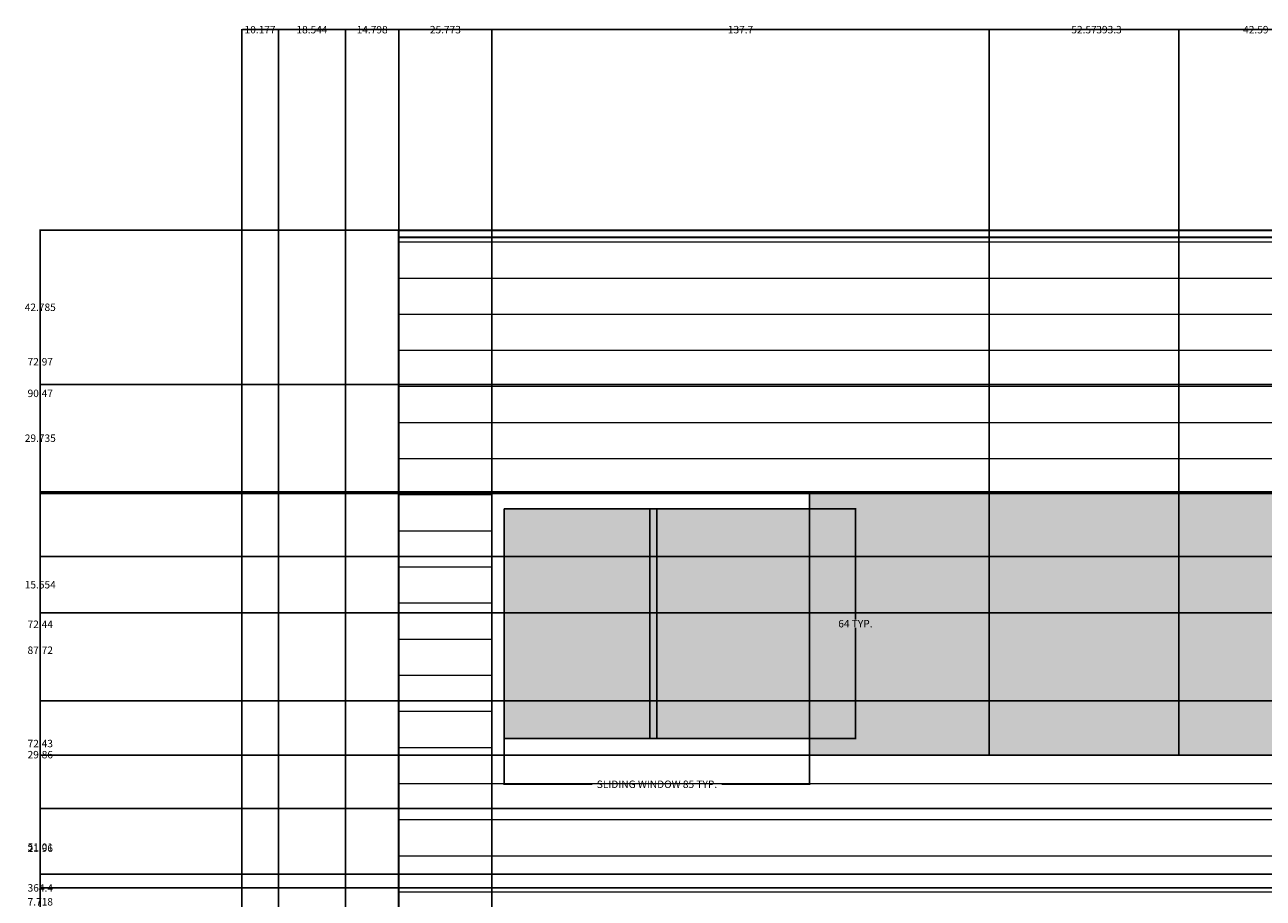
# Model space of a CAD drawing. Units: inches. Extents: x -30 to 1188, y 40 to 520.
# Tile 2 of 7: x -30 to 313, y 278 to 520. Entities that reach past the tile are written whole.
import ezdxf

# ---------------------------------------------------------------- set-up
doc = ezdxf.new("R2010")
doc.units = ezdxf.units.IN
doc.header["$MEASUREMENT"] = 0
for name, color, linetype, lineweight in [('A-ANNO-DIMS', 2, 'Continuous', 18), ('A-ELEV', 7, 'Continuous', 35), ('A-ELEV-PATT', 8, 'Continuous', 13), ('A-GLAZ', 4, 'Continuous', 25)]:
    doc.layers.add(name, color=color, linetype=linetype, lineweight=lineweight)
doc.styles.get("Standard").update_dxf_attribs({"font": 'arial.ttf'})
doc.dimstyles.get("Standard").update_dxf_attribs({"dimtxt": 2.0625, "dimasz": 0.18, "dimexe": 0.18, "dimexo": 0.0625, "dimgap": 0.09, "dimtad": 0, "dimtih": 1, "dimtoh": 1, "dimdec": 4, "dimzin": 0, "dimdsep": 46, "dimlunit": 4, "dimtxsty": 'Standard', "dimcen": 0.09, "dimadec": 0, "dimazin": 0, "dimtfac": 1, "dimtdec": 4, "dimtofl": 0, "dimtmove": 0, "dimatfit": 3, "dimfxl": 1, "dimtolj": 1, "dimtzin": 0, "dimarcsym": 0})

# ---------------------------------------------------------------- blocks, each defined once
blk = doc.blocks.new('WIN-SLIDING')
for p, q in [((40.27, 63.6), (40.27, 0)), ((42.27, 63.6), (42.27, 0))]:
    blk.add_line(p, q)
blk.add_lwpolyline([(0, 63.6), (84.55, 63.6), (84.55, 0), (0, 0)], close=True)
blk = doc.blocks.new('*D2')
at = {"layer": 'A-ANNO-DIMS', "color": 0, "lineweight": -2, "transparency": 16777216}
for p, q in [((102.87, 322.4), (102.87, 309.6)), ((187.42, 322.4), (187.42, 309.6)), ((103.05, 309.78), (127.15, 309.78)), ((187.24, 309.78), (163.13, 309.78))]:
    blk.add_line(p, q, dxfattribs=at)
at = {"layer": 'A-ANNO-DIMS', "color": 0, "transparency": 16777216}
for points in [[(103.05, 309.81), (103.05, 309.75), (102.87, 309.78)], [(187.24, 309.81), (187.24, 309.75), (187.42, 309.78)]]:
    blk.add_solid(points, dxfattribs=at)
at = {"layer": 'Defpoints', "color": 0, "transparency": 16777216}
for p in [(102.87, 322.46), (187.42, 322.46), (187.42, 309.78)]:
    blk.add_point(p, dxfattribs=at)
at = {"layer": 'A-ANNO-DIMS', "color": 0, "transparency": 16777216, "insert": (145.14, 309.78), "char_height": 2.0625, "attachment_point": 5}
blk.add_mtext('\\A1;SLIDING WINDOW 85 TYP.', dxfattribs=at)
blk = doc.blocks.new('*D3')
at = {"layer": 'A-ANNO-DIMS', "color": 0, "lineweight": -2, "transparency": 16777216}
for p, q in [((187.48, 386.06), (200.28, 386.06)), ((200.1, 385.88), (200.1, 355.4)), ((200.1, 322.64), (200.1, 353.12)), ((187.48, 322.46), (200.28, 322.46))]:
    blk.add_line(p, q, dxfattribs=at)
at = {"layer": 'A-ANNO-DIMS', "color": 0, "transparency": 16777216}
for points in [[(200.07, 385.88), (200.13, 385.88), (200.1, 386.06)], [(200.07, 322.64), (200.13, 322.64), (200.1, 322.46)]]:
    blk.add_solid(points, dxfattribs=at)
at = {"layer": 'Defpoints', "color": 0, "transparency": 16777216}
for p in [(187.42, 386.06), (200.1, 386.06), (187.42, 322.46)]:
    blk.add_point(p, dxfattribs=at)
at = {"layer": 'A-ANNO-DIMS', "color": 0, "transparency": 16777216, "insert": (200.1, 354.26), "char_height": 2.0625, "attachment_point": 5}
blk.add_mtext('\\A1;64 TYP.', dxfattribs=at)
blk = doc.blocks.new('*D5')
at = {"layer": 'A-ANNO-DIMS', "color": 0, "lineweight": -2, "transparency": 16777216}
for p, q in [((73.66, 463.36), (73.66, 518.97)), ((73.84, 518.79), (266.76, 518.79)), ((466.82, 518.79), (273.9, 518.79)), ((467, 463.36), (467, 518.97))]:
    blk.add_line(p, q, dxfattribs=at)
at = {"layer": 'A-ANNO-DIMS', "color": 0, "transparency": 16777216}
for points in [[(73.84, 518.82), (73.84, 518.76), (73.66, 518.79)], [(466.82, 518.82), (466.82, 518.76), (467, 518.79)]]:
    blk.add_solid(points, dxfattribs=at)
at = {"layer": 'Defpoints', "color": 0, "transparency": 16777216}
for p in [(467, 518.79), (73.66, 463.29), (467, 463.29)]:
    blk.add_point(p, dxfattribs=at)
at = {"layer": 'A-ANNO-DIMS', "color": 0, "transparency": 16777216, "insert": (270.33, 518.79), "char_height": 2.062, "attachment_point": 5}
blk.add_mtext('\\A1;393.3', dxfattribs=at)
blk = doc.blocks.new('*D10')
at = {"layer": 'A-ANNO-DIMS', "color": 0, "lineweight": -2, "transparency": 16777216}
for p, q in [((73.66, 242.93), (73.66, 518.97)), ((73.84, 518.79), (82.16, 518.79)), ((99.25, 518.79), (90.93, 518.79)), ((99.43, 242.93), (99.43, 518.97))]:
    blk.add_line(p, q, dxfattribs=at)
at = {"layer": 'A-ANNO-DIMS', "color": 0, "transparency": 16777216}
for points in [[(73.84, 518.82), (73.84, 518.76), (73.66, 518.79)], [(99.25, 518.82), (99.25, 518.76), (99.43, 518.79)]]:
    blk.add_solid(points, dxfattribs=at)
at = {"layer": 'Defpoints', "color": 0, "transparency": 16777216}
for p in [(99.43, 518.79), (73.66, 242.87), (99.43, 242.87)]:
    blk.add_point(p, dxfattribs=at)
at = {"layer": 'A-ANNO-DIMS', "color": 0, "transparency": 16777216, "insert": (86.54, 518.79), "char_height": 2.062, "attachment_point": 5}
blk.add_mtext('\\A1;25.773', dxfattribs=at)
blk = doc.blocks.new('*D12')
at = {"layer": 'A-ANNO-DIMS', "color": 0, "lineweight": -2, "transparency": 16777216}
for p, q in [((73.66, 410.93), (73.66, 518.97)), ((73.84, 518.79), (82.16, 518.79)), ((99.25, 518.79), (90.93, 518.79)), ((99.43, 390.39), (99.43, 518.97))]:
    blk.add_line(p, q, dxfattribs=at)
at = {"layer": 'A-ANNO-DIMS', "color": 0, "transparency": 16777216}
for points in [[(73.84, 518.82), (73.84, 518.76), (73.66, 518.79)], [(99.25, 518.82), (99.25, 518.76), (99.43, 518.79)]]:
    blk.add_solid(points, dxfattribs=at)
at = {"layer": 'Defpoints', "color": 0, "transparency": 16777216}
for p in [(99.43, 518.79), (73.66, 410.87), (99.43, 390.32)]:
    blk.add_point(p, dxfattribs=at)
at = {"layer": 'A-ANNO-DIMS', "color": 0, "transparency": 16777216, "insert": (86.54, 518.79), "char_height": 2.062, "attachment_point": 5}
blk.add_mtext('\\A1;25.773', dxfattribs=at)
blk = doc.blocks.new('*D13')
at = {"layer": 'A-ANNO-DIMS', "color": 0, "lineweight": -2, "transparency": 16777216}
for p, q in [((99.43, 390.39), (99.43, 518.97)), ((99.61, 518.79), (164.81, 518.79)), ((236.95, 518.79), (171.75, 518.79)), ((237.13, 390.39), (237.13, 518.97))]:
    blk.add_line(p, q, dxfattribs=at)
at = {"layer": 'A-ANNO-DIMS', "color": 0, "transparency": 16777216}
for points in [[(99.61, 518.82), (99.61, 518.76), (99.43, 518.79)], [(236.95, 518.82), (236.95, 518.76), (237.13, 518.79)]]:
    blk.add_solid(points, dxfattribs=at)
at = {"layer": 'Defpoints', "color": 0, "transparency": 16777216}
for p in [(237.13, 518.79), (99.43, 390.32), (237.13, 390.32)]:
    blk.add_point(p, dxfattribs=at)
at = {"layer": 'A-ANNO-DIMS', "color": 0, "transparency": 16777216, "insert": (168.28, 518.79), "char_height": 2.062, "attachment_point": 5}
blk.add_mtext('\\A1;137.7', dxfattribs=at)
blk = doc.blocks.new('*D14')
at = {"layer": 'A-ANNO-DIMS', "color": 0, "lineweight": -2, "transparency": 16777216}
for p, q in [((237.13, 390.39), (237.13, 518.97)), ((237.31, 518.79), (259.84, 518.79)), ((289.52, 518.79), (266.98, 518.79)), ((289.7, 390.39), (289.7, 518.97))]:
    blk.add_line(p, q, dxfattribs=at)
at = {"layer": 'A-ANNO-DIMS', "color": 0, "transparency": 16777216}
for points in [[(237.31, 518.82), (237.31, 518.76), (237.13, 518.79)], [(289.52, 518.82), (289.52, 518.76), (289.7, 518.79)]]:
    blk.add_solid(points, dxfattribs=at)
at = {"layer": 'Defpoints', "color": 0, "transparency": 16777216}
for p in [(289.7, 518.79), (237.13, 390.32), (289.7, 390.32)]:
    blk.add_point(p, dxfattribs=at)
at = {"layer": 'A-ANNO-DIMS', "color": 0, "transparency": 16777216, "insert": (263.41, 518.79), "char_height": 2.062, "attachment_point": 5}
blk.add_mtext('\\A1;52.57', dxfattribs=at)
blk = doc.blocks.new('*D15')
at = {"layer": 'A-ANNO-DIMS', "color": 0, "lineweight": -2, "transparency": 16777216}
for p, q in [((289.7, 390.39), (289.7, 518.97)), ((289.88, 518.79), (307.38, 518.79)), ((332.11, 518.79), (314.61, 518.79)), ((332.29, 385.96), (332.29, 518.97))]:
    blk.add_line(p, q, dxfattribs=at)
at = {"layer": 'A-ANNO-DIMS', "color": 0, "transparency": 16777216}
for points in [[(289.88, 518.82), (289.88, 518.76), (289.7, 518.79)], [(332.11, 518.82), (332.11, 518.76), (332.29, 518.79)]]:
    blk.add_solid(points, dxfattribs=at)
at = {"layer": 'Defpoints', "color": 0, "transparency": 16777216}
for p in [(332.29, 518.79), (289.7, 390.32), (332.29, 385.9)]:
    blk.add_point(p, dxfattribs=at)
at = {"layer": 'A-ANNO-DIMS', "color": 0, "transparency": 16777216, "insert": (310.99, 518.79), "char_height": 2.062, "attachment_point": 5}
blk.add_mtext('\\A1;42.59', dxfattribs=at)
blk = doc.blocks.new('*D18')
at = {"layer": 'A-ANNO-DIMS', "color": 0, "lineweight": -2, "transparency": 16777216}
for p, q in [((73.6, 463.29), (-25.83, 463.29)), ((-25.65, 463.11), (-25.65, 282.23)), ((-25.65, 99.05), (-25.65, 279.94)), ((30.08, 98.87), (-25.83, 98.87))]:
    blk.add_line(p, q, dxfattribs=at)
at = {"layer": 'A-ANNO-DIMS', "color": 0, "transparency": 16777216}
for points in [[(-25.68, 463.11), (-25.62, 463.11), (-25.65, 463.29)], [(-25.68, 99.05), (-25.62, 99.05), (-25.65, 98.87)]]:
    blk.add_solid(points, dxfattribs=at)
at = {"layer": 'Defpoints', "color": 0, "transparency": 16777216}
for p in [(-25.65, 463.29), (73.66, 463.29), (30.14, 98.87)]:
    blk.add_point(p, dxfattribs=at)
at = {"layer": 'A-ANNO-DIMS', "color": 0, "transparency": 16777216, "insert": (-25.65, 281.08), "char_height": 2.062, "attachment_point": 5}
blk.add_mtext('\\A1;364.4', dxfattribs=at)
blk = doc.blocks.new('*D21')
at = {"layer": 'A-ANNO-DIMS', "color": 0, "lineweight": -2, "transparency": 16777216}
for p, q in [((99.37, 390.32), (-25.83, 390.32)), ((-25.65, 390.14), (-25.65, 355.23)), ((-25.65, 318.06), (-25.65, 352.98)), ((99.37, 317.88), (-25.83, 317.88))]:
    blk.add_line(p, q, dxfattribs=at)
at = {"layer": 'A-ANNO-DIMS', "color": 0, "transparency": 16777216}
for points in [[(-25.68, 390.14), (-25.62, 390.14), (-25.65, 390.32)], [(-25.68, 318.06), (-25.62, 318.06), (-25.65, 317.88)]]:
    blk.add_solid(points, dxfattribs=at)
at = {"layer": 'Defpoints', "color": 0, "transparency": 16777216}
for p in [(99.43, 390.32), (-25.65, 317.88), (99.43, 317.88)]:
    blk.add_point(p, dxfattribs=at)
at = {"layer": 'A-ANNO-DIMS', "color": 0, "transparency": 16777216, "insert": (-25.65, 354.1), "char_height": 2.062, "attachment_point": 5}
blk.add_mtext('\\A1;72.44', dxfattribs=at)
blk = doc.blocks.new('*D24')
at = {"layer": 'A-ANNO-DIMS', "color": 0, "lineweight": -2, "transparency": 16777216}
for p, q in [((935.84, 463.29), (-25.83, 463.29)), ((-25.65, 463.11), (-25.65, 419.2)), ((-25.65, 373.01), (-25.65, 416.92)), ((980.66, 372.83), (-25.83, 372.83))]:
    blk.add_line(p, q, dxfattribs=at)
at = {"layer": 'A-ANNO-DIMS', "color": 0, "transparency": 16777216}
for points in [[(-25.68, 463.11), (-25.62, 463.11), (-25.65, 463.29)], [(-25.68, 373.01), (-25.62, 373.01), (-25.65, 372.83)]]:
    blk.add_solid(points, dxfattribs=at)
at = {"layer": 'Defpoints', "color": 0, "transparency": 16777216}
for p in [(-25.65, 463.29), (935.9, 463.29), (980.73, 372.83)]:
    blk.add_point(p, dxfattribs=at)
at = {"layer": 'A-ANNO-DIMS', "color": 0, "transparency": 16777216, "insert": (-25.65, 418.06), "char_height": 2.062, "attachment_point": 5}
blk.add_mtext('\\A1;90.47', dxfattribs=at)
blk = doc.blocks.new('*D32')
at = {"layer": 'A-ANNO-DIMS', "color": 0, "lineweight": -2, "transparency": 16777216}
for p, q in [((73.6, 463.29), (-25.83, 463.29)), ((-25.65, 463.11), (-25.65, 427.95)), ((-25.65, 390.5), (-25.65, 425.67)), ((99.37, 390.32), (-25.83, 390.32))]:
    blk.add_line(p, q, dxfattribs=at)
at = {"layer": 'A-ANNO-DIMS', "color": 0, "transparency": 16777216}
for points in [[(-25.68, 463.11), (-25.62, 463.11), (-25.65, 463.29)], [(-25.68, 390.5), (-25.62, 390.5), (-25.65, 390.32)]]:
    blk.add_solid(points, dxfattribs=at)
at = {"layer": 'Defpoints', "color": 0, "transparency": 16777216}
for p in [(73.66, 463.29), (-25.65, 390.32), (99.43, 390.32)]:
    blk.add_point(p, dxfattribs=at)
at = {"layer": 'A-ANNO-DIMS', "color": 0, "transparency": 16777216, "insert": (-25.65, 426.81), "char_height": 2.062, "attachment_point": 5}
blk.add_mtext('\\A1;72.97', dxfattribs=at)
blk = doc.blocks.new('*D33')
at = {"layer": 'A-ANNO-DIMS', "color": 0, "lineweight": -2, "transparency": 16777216}
for p, q in [((99.37, 317.88), (-25.83, 317.88)), ((-25.65, 317.7), (-25.65, 293.52)), ((-25.65, 267.05), (-25.65, 291.23)), ((73.6, 266.87), (-25.83, 266.87))]:
    blk.add_line(p, q, dxfattribs=at)
at = {"layer": 'A-ANNO-DIMS', "color": 0, "transparency": 16777216}
for points in [[(-25.68, 317.7), (-25.62, 317.7), (-25.65, 317.88)], [(-25.68, 267.05), (-25.62, 267.05), (-25.65, 266.87)]]:
    blk.add_solid(points, dxfattribs=at)
at = {"layer": 'Defpoints', "color": 0, "transparency": 16777216}
for p in [(99.43, 317.88), (-25.65, 266.87), (73.66, 266.87)]:
    blk.add_point(p, dxfattribs=at)
at = {"layer": 'A-ANNO-DIMS', "color": 0, "transparency": 16777216, "insert": (-25.65, 292.38), "char_height": 2.062, "attachment_point": 5}
blk.add_mtext('\\A1;51.01', dxfattribs=at)
blk = doc.blocks.new('*D41')
at = {"layer": 'A-ANNO-DIMS', "color": 0, "lineweight": -2, "transparency": 16777216}
for p, q in [((654.97, 463.29), (-25.83, 463.29)), ((-25.65, 463.11), (-25.65, 443.04)), ((-25.65, 420.69), (-25.65, 440.76)), ((654.97, 420.51), (-25.83, 420.51))]:
    blk.add_line(p, q, dxfattribs=at)
at = {"layer": 'A-ANNO-DIMS', "color": 0, "transparency": 16777216}
for points in [[(-25.68, 463.11), (-25.62, 463.11), (-25.65, 463.29)], [(-25.68, 420.69), (-25.62, 420.69), (-25.65, 420.51)]]:
    blk.add_solid(points, dxfattribs=at)
at = {"layer": 'Defpoints', "color": 0, "transparency": 16777216}
for p in [(655.03, 463.29), (-25.65, 420.51), (655.03, 420.51)]:
    blk.add_point(p, dxfattribs=at)
at = {"layer": 'A-ANNO-DIMS', "color": 0, "transparency": 16777216, "insert": (-25.65, 441.9), "char_height": 2.062, "attachment_point": 5}
blk.add_mtext('\\A1;42.785', dxfattribs=at)
blk = doc.blocks.new('*D45')
at = {"layer": 'A-ANNO-DIMS', "color": 0, "lineweight": -2, "transparency": 16777216}
for p, q in [((945.03, 284.84), (-25.83, 284.84)), ((-25.65, 284.66), (-25.65, 273.81)), ((-25.65, 260.67), (-25.65, 271.52)), ((935.84, 260.49), (-25.83, 260.49))]:
    blk.add_line(p, q, dxfattribs=at)
at = {"layer": 'A-ANNO-DIMS', "color": 0, "transparency": 16777216}
for points in [[(-25.68, 284.66), (-25.62, 284.66), (-25.65, 284.84)], [(-25.68, 260.67), (-25.62, 260.67), (-25.65, 260.49)]]:
    blk.add_solid(points, dxfattribs=at)
at = {"layer": 'Defpoints', "color": 0, "transparency": 16777216}
for p in [(945.1, 284.84), (-25.65, 260.49), (935.9, 260.49)]:
    blk.add_point(p, dxfattribs=at)
at = {"layer": 'A-ANNO-DIMS', "color": 0, "transparency": 16777216, "insert": (-25.65, 272.67), "char_height": 2.062, "attachment_point": 5}
blk.add_mtext('\\A1;24.35', dxfattribs=at)
blk = doc.blocks.new('*D46')
at = {"layer": 'A-ANNO-DIMS', "color": 0, "lineweight": -2, "transparency": 16777216}
for p, q in [((945.03, 357.27), (-25.83, 357.27)), ((-25.65, 357.09), (-25.65, 322.2)), ((-25.65, 285.02), (-25.65, 319.91)), ((945.03, 284.84), (-25.83, 284.84))]:
    blk.add_line(p, q, dxfattribs=at)
at = {"layer": 'A-ANNO-DIMS', "color": 0, "transparency": 16777216}
for points in [[(-25.68, 357.09), (-25.62, 357.09), (-25.65, 357.27)], [(-25.68, 285.02), (-25.62, 285.02), (-25.65, 284.84)]]:
    blk.add_solid(points, dxfattribs=at)
at = {"layer": 'Defpoints', "color": 0, "transparency": 16777216}
for p in [(-25.65, 357.27), (945.1, 357.27), (945.1, 284.84)]:
    blk.add_point(p, dxfattribs=at)
at = {"layer": 'A-ANNO-DIMS', "color": 0, "transparency": 16777216, "insert": (-25.65, 321.06), "char_height": 2.062, "attachment_point": 5}
blk.add_mtext('\\A1;72.43', dxfattribs=at)
blk = doc.blocks.new('*D47')
at = {"layer": 'A-ANNO-DIMS', "color": 0, "lineweight": -2, "transparency": 16777216}
for p, q in [((935.84, 372.83), (-25.83, 372.83)), ((-25.65, 372.65), (-25.65, 366.19)), ((-25.65, 357.45), (-25.65, 363.91)), ((945.03, 357.27), (-25.83, 357.27))]:
    blk.add_line(p, q, dxfattribs=at)
at = {"layer": 'A-ANNO-DIMS', "color": 0, "transparency": 16777216}
for points in [[(-25.68, 372.65), (-25.62, 372.65), (-25.65, 372.83)], [(-25.68, 357.45), (-25.62, 357.45), (-25.65, 357.27)]]:
    blk.add_solid(points, dxfattribs=at)
at = {"layer": 'Defpoints', "color": 0, "transparency": 16777216}
for p in [(-25.65, 372.83), (935.9, 372.83), (945.1, 357.27)]:
    blk.add_point(p, dxfattribs=at)
at = {"layer": 'A-ANNO-DIMS', "color": 0, "transparency": 16777216, "insert": (-25.65, 365.05), "char_height": 2.062, "attachment_point": 5}
blk.add_mtext('\\A1;15.554', dxfattribs=at)
blk = doc.blocks.new('*D52')
at = {"layer": 'A-ANNO-DIMS', "color": 0, "lineweight": -2, "transparency": 16777216}
for p, q in [((30.14, 178.91), (30.14, 518.97)), ((30.32, 518.79), (30.95, 518.79)), ((40.14, 518.79), (39.5, 518.79)), ((40.32, 178.91), (40.32, 518.97))]:
    blk.add_line(p, q, dxfattribs=at)
at = {"layer": 'A-ANNO-DIMS', "color": 0, "transparency": 16777216}
for points in [[(30.32, 518.82), (30.32, 518.76), (30.14, 518.79)], [(40.14, 518.82), (40.14, 518.76), (40.32, 518.79)]]:
    blk.add_solid(points, dxfattribs=at)
at = {"layer": 'Defpoints', "color": 0, "transparency": 16777216}
for p in [(40.32, 518.79), (30.14, 178.84), (40.32, 178.84)]:
    blk.add_point(p, dxfattribs=at)
at = {"layer": 'A-ANNO-DIMS', "color": 0, "transparency": 16777216, "insert": (35.23, 518.79), "char_height": 2.062, "attachment_point": 5}
blk.add_mtext('\\A1;10.177', dxfattribs=at)
blk = doc.blocks.new('*D53')
at = {"layer": 'A-ANNO-DIMS', "color": 0, "lineweight": -2, "transparency": 16777216}
for p, q in [((40.32, 178.91), (40.32, 518.97)), ((40.5, 518.79), (45.32, 518.79)), ((58.68, 518.79), (53.86, 518.79)), ((58.86, 178.91), (58.86, 518.97))]:
    blk.add_line(p, q, dxfattribs=at)
at = {"layer": 'A-ANNO-DIMS', "color": 0, "transparency": 16777216}
for points in [[(40.5, 518.82), (40.5, 518.76), (40.32, 518.79)], [(58.68, 518.82), (58.68, 518.76), (58.86, 518.79)]]:
    blk.add_solid(points, dxfattribs=at)
at = {"layer": 'Defpoints', "color": 0, "transparency": 16777216}
for p in [(58.86, 518.79), (40.32, 178.84), (58.86, 178.84)]:
    blk.add_point(p, dxfattribs=at)
at = {"layer": 'A-ANNO-DIMS', "color": 0, "transparency": 16777216, "insert": (49.59, 518.79), "char_height": 2.062, "attachment_point": 5}
blk.add_mtext('\\A1;18.544', dxfattribs=at)
blk = doc.blocks.new('*D54')
at = {"layer": 'A-ANNO-DIMS', "color": 0, "lineweight": -2, "transparency": 16777216}
for p, q in [((58.86, 178.91), (58.86, 518.97)), ((59.04, 518.79), (61.98, 518.79)), ((73.48, 518.79), (70.54, 518.79)), ((73.66, 178.91), (73.66, 518.97))]:
    blk.add_line(p, q, dxfattribs=at)
at = {"layer": 'A-ANNO-DIMS', "color": 0, "transparency": 16777216}
for points in [[(59.04, 518.82), (59.04, 518.76), (58.86, 518.79)], [(73.48, 518.82), (73.48, 518.76), (73.66, 518.79)]]:
    blk.add_solid(points, dxfattribs=at)
at = {"layer": 'Defpoints', "color": 0, "transparency": 16777216}
for p in [(73.66, 518.79), (58.86, 178.84), (73.66, 178.84)]:
    blk.add_point(p, dxfattribs=at)
at = {"layer": 'A-ANNO-DIMS', "color": 0, "transparency": 16777216, "insert": (66.26, 518.79), "char_height": 2.062, "attachment_point": 5}
blk.add_mtext('\\A1;14.798', dxfattribs=at)
blk = doc.blocks.new('*D57')
at = {"layer": 'A-ANNO-DIMS', "color": 0, "lineweight": -2, "transparency": 16777216}
for p, q in [((466.93, 281.09), (-25.83, 281.09)), ((-25.65, 280.91), (-25.65, 278.38)), ((-25.65, 273.56), (-25.65, 276.09)), ((466.76, 273.38), (-25.83, 273.38))]:
    blk.add_line(p, q, dxfattribs=at)
at = {"layer": 'A-ANNO-DIMS', "color": 0, "transparency": 16777216}
for points in [[(-25.68, 280.91), (-25.62, 280.91), (-25.65, 281.09)], [(-25.68, 273.56), (-25.62, 273.56), (-25.65, 273.38)]]:
    blk.add_solid(points, dxfattribs=at)
at = {"layer": 'Defpoints', "color": 0, "transparency": 16777216}
for p in [(-25.65, 281.09), (467, 281.09), (466.83, 273.38)]:
    blk.add_point(p, dxfattribs=at)
at = {"layer": 'A-ANNO-DIMS', "color": 0, "transparency": 16777216, "insert": (-25.65, 277.23), "char_height": 2.062, "attachment_point": 5}
blk.add_mtext('\\A1;7.718', dxfattribs=at)
blk = doc.blocks.new('*D58')
at = {"layer": 'A-ANNO-DIMS', "color": 0, "lineweight": -2, "transparency": 16777216}
for p, q in [((466.93, 303.05), (-25.83, 303.05)), ((-25.65, 302.87), (-25.65, 293.22)), ((-25.65, 281.27), (-25.65, 290.93)), ((466.93, 281.09), (-25.83, 281.09))]:
    blk.add_line(p, q, dxfattribs=at)
at = {"layer": 'A-ANNO-DIMS', "color": 0, "transparency": 16777216}
for points in [[(-25.68, 302.87), (-25.62, 302.87), (-25.65, 303.05)], [(-25.68, 281.27), (-25.62, 281.27), (-25.65, 281.09)]]:
    blk.add_solid(points, dxfattribs=at)
at = {"layer": 'Defpoints', "color": 0, "transparency": 16777216}
for p in [(-25.65, 303.05), (467, 303.05), (467, 281.09)]:
    blk.add_point(p, dxfattribs=at)
at = {"layer": 'A-ANNO-DIMS', "color": 0, "transparency": 16777216, "insert": (-25.65, 292.07), "char_height": 2.062, "attachment_point": 5}
blk.add_mtext('\\A1;21.96', dxfattribs=at)
blk = doc.blocks.new('*D59')
at = {"layer": 'A-ANNO-DIMS', "color": 0, "lineweight": -2, "transparency": 16777216}
for p, q in [((466.93, 390.77), (-25.83, 390.77)), ((-25.65, 390.59), (-25.65, 348.06)), ((-25.65, 303.23), (-25.65, 345.77)), ((466.93, 303.05), (-25.83, 303.05))]:
    blk.add_line(p, q, dxfattribs=at)
at = {"layer": 'A-ANNO-DIMS', "color": 0, "transparency": 16777216}
for points in [[(-25.68, 390.59), (-25.62, 390.59), (-25.65, 390.77)], [(-25.68, 303.23), (-25.62, 303.23), (-25.65, 303.05)]]:
    blk.add_solid(points, dxfattribs=at)
at = {"layer": 'Defpoints', "color": 0, "transparency": 16777216}
for p in [(-25.65, 390.77), (467, 390.77), (467, 303.05)]:
    blk.add_point(p, dxfattribs=at)
at = {"layer": 'A-ANNO-DIMS', "color": 0, "transparency": 16777216, "insert": (-25.65, 346.91), "char_height": 2.062, "attachment_point": 5}
blk.add_mtext('\\A1;87.72', dxfattribs=at)
blk = doc.blocks.new('*D60')
at = {"layer": 'A-ANNO-DIMS', "color": 0, "lineweight": -2, "transparency": 16777216}
for p, q in [((466.93, 420.51), (-25.83, 420.51)), ((-25.65, 420.33), (-25.65, 406.78)), ((-25.65, 390.95), (-25.65, 404.5)), ((466.93, 390.77), (-25.83, 390.77))]:
    blk.add_line(p, q, dxfattribs=at)
at = {"layer": 'A-ANNO-DIMS', "color": 0, "transparency": 16777216}
for points in [[(-25.68, 420.33), (-25.62, 420.33), (-25.65, 420.51)], [(-25.68, 390.95), (-25.62, 390.95), (-25.65, 390.77)]]:
    blk.add_solid(points, dxfattribs=at)
at = {"layer": 'Defpoints', "color": 0, "transparency": 16777216}
for p in [(-25.65, 420.51), (467, 420.51), (467, 390.77)]:
    blk.add_point(p, dxfattribs=at)
at = {"layer": 'A-ANNO-DIMS', "color": 0, "transparency": 16777216, "insert": (-25.65, 405.64), "char_height": 2.062, "attachment_point": 5}
blk.add_mtext('\\A1;29.735', dxfattribs=at)
blk = doc.blocks.new('*D69')
at = {"layer": 'A-ANNO-DIMS', "color": 0, "lineweight": -2, "transparency": 16777216}
for p, q in [((530.66, 332.91), (-25.83, 332.91)), ((-25.65, 332.73), (-25.65, 319.13)), ((-25.65, 303.23), (-25.65, 316.84)), ((520.94, 303.05), (-25.83, 303.05))]:
    blk.add_line(p, q, dxfattribs=at)
at = {"layer": 'A-ANNO-DIMS', "color": 0, "transparency": 16777216}
for points in [[(-25.68, 332.73), (-25.62, 332.73), (-25.65, 332.91)], [(-25.68, 303.23), (-25.62, 303.23), (-25.65, 303.05)]]:
    blk.add_solid(points, dxfattribs=at)
at = {"layer": 'Defpoints', "color": 0, "transparency": 16777216}
for p in [(-25.65, 332.91), (530.73, 332.91), (521.01, 303.05)]:
    blk.add_point(p, dxfattribs=at)
at = {"layer": 'A-ANNO-DIMS', "color": 0, "transparency": 16777216, "insert": (-25.65, 317.98), "char_height": 2.062, "attachment_point": 5}
blk.add_mtext('\\A1;29.86', dxfattribs=at)
blk = doc.blocks.new('*D74')
at = {"layer": 'A-ANNO-DIMS', "color": 0, "lineweight": -2, "transparency": 16777216}
for p, q in [((30.14, 98.93), (30.14, 518.97)), ((30.32, 518.79), (574.32, 518.79)), ((1128.07, 518.79), (584.07, 518.79)), ((1128.25, 117.62), (1128.25, 518.97))]:
    blk.add_line(p, q, dxfattribs=at)
at = {"layer": 'A-ANNO-DIMS', "color": 0, "transparency": 16777216}
for points in [[(30.32, 518.82), (30.32, 518.76), (30.14, 518.79)], [(1128.07, 518.82), (1128.07, 518.76), (1128.25, 518.79)]]:
    blk.add_solid(points, dxfattribs=at)
at = {"layer": 'Defpoints', "color": 0, "transparency": 16777216}
for p in [(1128.25, 518.79), (1128.25, 117.56), (30.14, 98.87)]:
    blk.add_point(p, dxfattribs=at)
at = {"layer": 'A-ANNO-DIMS', "color": 0, "transparency": 16777216, "insert": (579.19, 518.79), "char_height": 2.0625, "attachment_point": 5}
blk.add_mtext('\\A1;1098.11', dxfattribs=at)

msp = doc.modelspace()

# ---------------------------------------------------------------- hatches: boundary and pattern name
at = {"layer": 'A-ELEV-PATT'}
h = msp.add_hatch(dxfattribs=at)
h.set_pattern_fill('ANSI31', color=256, scale=80, angle=135)
h.paths.add_polyline_path([(935.904, 461.2934), (655.0318, 461.2934), (655.0318, 408.0708), (655.0318, 380.8615), (798.3036, 380.8615), (798.3036, 314.3348), (655.0318, 314.3348), (655.0318, 303.0545), (655.0318, 122.8714), (744.4225, 122.8714), (796.5546, 122.8714), (935.904, 122.8714), (935.904, 203.8438), (792.6322, 203.8438), (792.6322, 270.3705), (935.904, 270.3705), (935.904, 372.8284)])
h.paths.add_polyline_path([(466.9951, 434.8714), (466.9951, 461.2934), (73.6582, 461.2934), (73.6582, 434.8714), (73.6582, 410.8714), (73.6582, 266.8714), (382.4247, 266.8714), (466.9951, 266.8714)])
h.paths.add_polyline_path([(422.6392, 390.3227), (422.6392, 317.8826), (99.4312, 317.8826), (99.4312, 390.3227)], flags=16)
h.paths.add_polyline_path([(416.8376, 385.9009), (416.8376, 322.3026), (332.2885, 322.3026), (332.2885, 385.9009)], flags=0)
h.paths.add_polyline_path([(187.4151, 386.0591), (187.4151, 322.4608), (102.866, 322.4608), (102.866, 386.0591)], flags=0)
h = msp.add_hatch(color=256, dxfattribs=at)
h.dxf.hatch_style = 1
h.paths.add_polyline_path([(521.0073, 390.7733), (466.9951, 390.7733), (466.9951, 303.0545), (521.0073, 303.0545)])
h.paths.add_polyline_path([(588.0971, 390.7733), (523.0073, 390.7733), (523.0073, 303.0545), (588.0971, 303.0545)])
h.paths.add_polyline_path([(579.9749, 370.1304), (579.9749, 332.9128), (530.7254, 332.9128), (530.7254, 370.1304)], flags=16)
h.paths.add_polyline_path([(577.9749, 368.1304), (577.9749, 334.9128), (532.7254, 334.9128), (532.7254, 368.1304)], flags=0)
h.paths.add_polyline_path([(655.0318, 390.7733), (590.0971, 390.7733), (590.0971, 303.0545), (655.0318, 303.0545)])
h.paths.add_polyline_path([(577.9749, 368.1304), (532.7254, 368.1304), (532.7254, 334.9128), (577.9749, 334.9128)], flags=0)
h.paths.add_polyline_path([(416.8376, 385.9009), (374.5631, 385.9009), (374.5631, 322.3026), (416.8376, 322.3026)])
h.paths.add_polyline_path([(372.5631, 385.9009), (332.2885, 385.9009), (332.2885, 322.3026), (372.5631, 322.3026)])
h.paths.add_polyline_path([(187.4151, 386.0591), (102.866, 386.0591), (102.866, 322.4608), (187.4151, 322.4608)])
h.paths.add_polyline_path([(697.0557, 378.8615), (657.0318, 378.8615), (657.0318, 316.3348), (697.0557, 316.3348)])
h.paths.add_polyline_path([(746.916, 378.8615), (699.0557, 378.8615), (699.0557, 316.3348), (746.916, 316.3348)])
h.paths.add_polyline_path([(796.3036, 378.8615), (748.916, 378.8615), (748.916, 316.3348), (796.3036, 316.3348)])
h.paths.add_polyline_path([(884.5164, 268.3705), (836.6561, 268.3705), (836.6561, 205.8438), (884.5164, 205.8438)])
h.paths.add_polyline_path([(834.6561, 268.3705), (794.6322, 268.3705), (794.6322, 205.8438), (834.6561, 205.8438)])
h.paths.add_polyline_path([(967.928, 357.2748), (945.0964, 357.2748), (945.0964, 284.8425), (967.928, 284.8425)])
h = msp.add_hatch(color=256, dxfattribs=at)
h.dxf.hatch_style = 1
h.paths.add_polyline_path([(237.1312, 390.3227), (187.4151, 390.3227), (187.4151, 386.0591), (187.4151, 322.4608), (187.4151, 317.8826), (237.1312, 317.8826)])
h.paths.add_polyline_path([(289.6973, 390.3227), (237.1312, 390.3227), (237.1312, 317.8826), (289.6973, 317.8826)])
h.paths.add_polyline_path([(422.6392, 390.3227), (289.6973, 390.3227), (289.6973, 317.8826), (422.6392, 317.8826)])
h.paths.add_polyline_path([(332.2885, 385.9009), (416.8376, 385.9009), (416.8376, 322.3026), (332.2885, 322.3026)], flags=16)
h.paths.add_polyline_path([(520.8377, 255.4488), (468.8255, 255.4488), (468.8255, 208.218), (520.8377, 208.218)])
h.paths.add_polyline_path([(573.9028, 245.1654), (576.7826, 245.1654), (576.7826, 208.218), (587.9675, 208.218), (587.9675, 255.4488), (522.8377, 255.4488), (522.8377, 208.218), (573.9028, 208.218)])
h.paths.add_polyline_path([(652.8622, 255.4488), (589.9675, 255.4488), (589.9675, 208.218), (652.8622, 208.218)])
h.paths.add_polyline_path([(652.8622, 206.218), (589.9675, 206.218), (589.9675, 142.7981), (652.8622, 142.7981)])
h.paths.add_polyline_path([(573.9028, 206.218), (522.8377, 206.218), (522.8377, 142.7981), (587.9675, 142.7981), (587.9675, 206.218), (576.7826, 206.218), (576.7826, 153.0843), (573.9028, 153.0843)])
h.paths.add_polyline_path([(520.8377, 206.218), (468.8255, 206.218), (468.8255, 142.7981), (520.8377, 142.7981)])
h.paths.add_polyline_path([(520.8377, 271.3754), (468.8255, 271.3754), (468.8255, 255.4488), (520.8377, 255.4488)])
h.paths.add_polyline_path([(587.9675, 271.3754), (522.8377, 271.3754), (522.8377, 255.4488), (587.9675, 255.4488)])
h.paths.add_polyline_path([(652.8622, 271.3754), (589.9675, 271.3754), (589.9675, 255.4488), (652.8622, 255.4488)])
h.paths.add_polyline_path([(935.904, 270.3705), (886.5164, 270.3705), (886.5164, 268.3705), (886.5164, 205.8438), (886.5164, 203.8438), (935.904, 203.8438)])
h.paths.add_polyline_path([(978.7252, 275.3408), (937.904, 275.3408), (937.904, 262.4906), (978.7252, 262.4906)])
h.paths.add_polyline_path([(978.7252, 370.8284), (937.904, 370.8284), (937.904, 275.3408), (978.7252, 275.3408)])
h.paths.add_polyline_path([(967.928, 284.8425), (945.0964, 284.8425), (945.0964, 357.2748), (967.928, 357.2748)], flags=16)

# ---------------------------------------------------------------- linework, layer by layer
at = {"layer": 'A-ELEV'}
for p, q in [((73.6582, 463.2934), (466.9951, 463.2934)), ((73.6582, 434.8714), (73.6582, 463.2934)), ((73.6582, 461.2934), (466.9951, 461.2934)), ((73.6582, 410.8714), (73.6582, 434.8714)), ((73.6582, 266.8714), (73.6582, 410.8714))]:
    msp.add_line(p, q, dxfattribs=at)
at = {"layer": 'A-GLAZ'}
for p, q in [((187.4151, 386.0591), (187.4151, 390.3227)), ((237.1312, 390.3227), (237.1312, 317.8826)), ((289.6973, 390.3227), (289.6973, 317.8826)), ((187.4151, 322.4608), (187.4151, 317.8826))]:
    msp.add_line(p, q, dxfattribs=at)
msp.add_lwpolyline([(99.4312, 390.3227), (422.6392, 390.3227), (422.6392, 317.8826), (99.4312, 317.8826)], close=True, dxfattribs=at)

# ---------------------------------------------------------------- block references
msp.add_blockref('WIN-SLIDING', (102.866, 322.461), dxfattribs=at)

# ---------------------------------------------------------------- dimensions: what is measured, and where the dimension line sits
at = {"layer": 'A-ANNO-DIMS'}
for base, p1, p2, override, picture, middle in [((40.3164, 518.7934), (30.1395, 178.8431), (40.3164, 178.8431), {"dimdec": 3, "dimlfac": 1, "dimrnd": 0, "dimzin": 0, "dimdsep": 46, "dimlunit": 2}, '*D52', (35.228, 518.7934)), ((1128.2474, 518.7934), (30.1395, 98.8714), (1128.2474, 117.5588), {"dimdec": 2, "dimlfac": 1, "dimrnd": 0, "dimzin": 0, "dimdsep": 46, "dimlunit": 2}, '*D74', (579.1935, 518.7934)), ((58.8603, 518.7934), (40.3164, 178.8431), (58.8603, 178.8431), {"dimdec": 3, "dimlfac": 1, "dimrnd": 0, "dimzin": 0, "dimdsep": 46, "dimlunit": 2}, '*D53', (49.5883, 518.7934)), ((73.6582, 518.7934), (58.8603, 178.8431), (73.6582, 178.8431), {"dimdec": 3, "dimlfac": 1, "dimrnd": 0, "dimzin": 0, "dimdsep": 46, "dimlunit": 2}, '*D54', (66.2592, 518.7934)), ((466.9951, 518.7934), (73.6582, 463.2934), (466.9951, 463.2934), {"dimdec": 1, "dimlfac": 1, "dimrnd": 0, "dimzin": 0, "dimdsep": 46, "dimlunit": 2}, '*D5', (270.3266, 518.7934)), ((99.4312, 518.7934), (73.6582, 242.8714), (99.4312, 242.8714), {"dimdec": 3, "dimlfac": 1, "dimrnd": 0, "dimzin": 0, "dimdsep": 46, "dimlunit": 2}, '*D10', (86.5447, 518.7934)), ((99.4312, 518.7934), (73.6582, 410.8714), (99.4312, 390.3227), {"dimdec": 3, "dimlfac": 1, "dimrnd": 0, "dimzin": 0, "dimdsep": 46, "dimlunit": 2}, '*D12', (86.5447, 518.7934)), ((237.1312, 518.7934), (99.4312, 390.3227), (237.1312, 390.3227), {"dimdec": 1, "dimlfac": 1, "dimrnd": 0, "dimzin": 0, "dimdsep": 46, "dimlunit": 2}, '*D13', (168.2812, 518.7934)), ((289.6973, 518.7934), (237.1312, 390.3227), (289.6973, 390.3227), {"dimdec": 2, "dimlfac": 1, "dimrnd": 0, "dimzin": 0, "dimdsep": 46, "dimlunit": 2}, '*D14', (263.4142, 518.7934)), ((332.2885, 518.7934), (289.6973, 390.3227), (332.2885, 385.9009), {"dimdec": 2, "dimlfac": 1, "dimrnd": 0, "dimzin": 0, "dimdsep": 46, "dimlunit": 2}, '*D15', (310.9929, 518.7934))]:
    dim = msp.add_linear_dim(base=base, p1=p1, p2=p2, dimstyle='Standard', override=override, dxfattribs=at)
    dim.commit()
    dim.dimension.update_dxf_attribs({"geometry": picture, "text_midpoint": middle})
for base, p1, p2, override, picture, middle in [((-25.6484, 420.5083), (655.0318, 463.2934), (655.0318, 420.5083), {"dimdec": 3, "dimlfac": 1, "dimrnd": 0, "dimzin": 0, "dimdsep": 46, "dimlunit": 2}, '*D41', (-25.6484, 441.9009)), ((-25.6484, 463.2934), (30.1395, 98.8714), (73.6582, 463.2934), {"dimdec": 1, "dimlfac": 1, "dimrnd": 0, "dimzin": 0, "dimdsep": 46, "dimlunit": 2}, '*D18', (-25.6484, 281.0824)), ((-25.64838, 463.29342), (980.72519, 372.8284), (935.90404, 463.29342), {"dimdec": 2, "dimlfac": 1, "dimrnd": 0, "dimzin": 0, "dimdsep": 46, "dimlunit": 2}, '*D24', (-25.64838, 418.06091)), ((-25.6484, 390.3227), (73.6582, 463.2934), (99.4312, 390.3227), {"dimdec": 2, "dimlfac": 1, "dimrnd": 0, "dimzin": 0, "dimdsep": 46, "dimlunit": 2}, '*D32', (-25.6484, 426.8081)), ((-25.6484, 420.5083), (466.9951, 390.7733), (466.9951, 420.5083), {"dimdec": 3, "dimlfac": 1, "dimrnd": 0, "dimzin": 0, "dimdsep": 46, "dimlunit": 2}, '*D60', (-25.6484, 405.6408)), ((-25.6484, 390.7733), (466.9951, 303.0545), (466.9951, 390.7733), {"dimdec": 2, "dimlfac": 1, "dimrnd": 0, "dimzin": 0, "dimdsep": 46, "dimlunit": 2}, '*D59', (-25.6484, 346.9139)), ((-25.6484, 317.8826), (99.4312, 390.3227), (99.4312, 317.8826), {"dimdec": 2, "dimlfac": 1, "dimrnd": 0, "dimzin": 0, "dimdsep": 46, "dimlunit": 2}, '*D21', (-25.6484, 354.1027)), ((-25.6484, 372.8284), (945.0964, 357.2748), (935.904, 372.8284), {"dimdec": 3, "dimlfac": 1, "dimrnd": 0, "dimzin": 0, "dimdsep": 46, "dimlunit": 2}, '*D47', (-25.6484, 365.0516)), ((-25.6484, 357.2748), (945.0964, 284.8425), (945.0964, 357.2748), {"dimdec": 2, "dimlfac": 1, "dimrnd": 0, "dimzin": 0, "dimdsep": 46, "dimlunit": 2}, '*D46', (-25.6484, 321.0586)), ((-25.6484, 332.9128), (521.0073, 303.0545), (530.7254, 332.9128), {"dimdec": 2, "dimlfac": 1, "dimrnd": 0, "dimzin": 0, "dimdsep": 46, "dimlunit": 2}, '*D69', (-25.6484, 317.9837)), ((-25.6484, 266.8714), (99.4312, 317.8826), (73.6582, 266.8714), {"dimdec": 2, "dimlfac": 1, "dimrnd": 0, "dimzin": 0, "dimdsep": 46, "dimlunit": 2}, '*D33', (-25.6484, 292.377)), ((-25.6484, 303.0545), (466.9951, 281.0934), (466.9951, 303.0545), {"dimdec": 2, "dimlfac": 1, "dimrnd": 0, "dimzin": 0, "dimdsep": 46, "dimlunit": 2}, '*D58', (-25.6484, 292.074)), ((-25.6484, 260.4906), (945.0964, 284.8425), (935.904, 260.4906), {"dimdec": 2, "dimlfac": 1, "dimrnd": 0, "dimzin": 0, "dimdsep": 46, "dimlunit": 2}, '*D45', (-25.6484, 272.6666)), ((-25.6484, 281.0934), (466.8255, 273.3754), (466.9951, 281.0934), {"dimdec": 3, "dimlfac": 1, "dimrnd": 0, "dimzin": 0, "dimdsep": 46, "dimlunit": 2}, '*D57', (-25.6484, 277.2344))]:
    dim = msp.add_linear_dim(base=base, p1=p1, p2=p2, angle=90, dimstyle='Standard', override=override, dxfattribs=at)
    dim.commit()
    dim.dimension.update_dxf_attribs({"geometry": picture, "text_midpoint": middle})
dim = msp.add_linear_dim(base=(200.0974, 386.0591), p1=(187.4151, 322.4608), p2=(187.4151, 386.0591), angle=90, text='<> TYP.', dimstyle='Standard', override={"dimdec": 0, "dimlfac": 1, "dimrnd": 0, "dimzin": 0, "dimdsep": 46, "dimlunit": 2}, dxfattribs=at)
dim.commit()
dim.dimension.update_dxf_attribs({"geometry": '*D3', "text_midpoint": (200.0974, 354.26)})
dim = msp.add_linear_dim(base=(187.4151, 309.7784), p1=(102.866, 322.4608), p2=(187.4151, 322.4608), text='SLIDING WINDOW <> TYP.', dimstyle='Standard', override={"dimdec": 0, "dimlfac": 1, "dimrnd": 0, "dimzin": 0, "dimdsep": 46, "dimlunit": 2}, dxfattribs=at)
dim.commit()
dim.dimension.update_dxf_attribs({"geometry": '*D2', "text_midpoint": (145.1405, 309.7784)})

doc.saveas('drawing.dxf')
